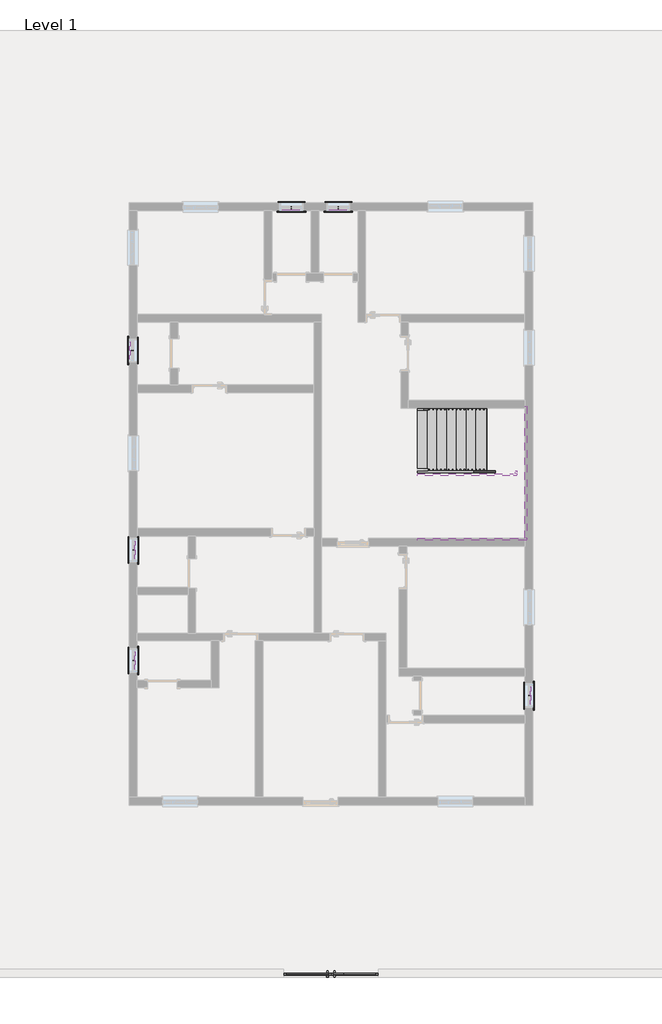
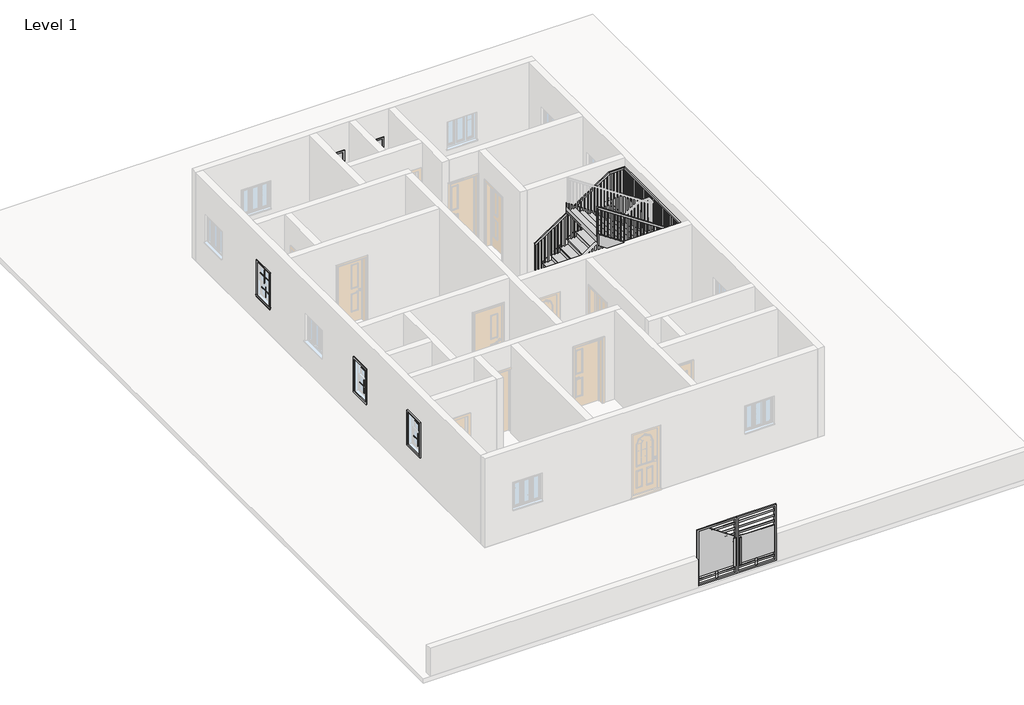
# One storey, part 3 of 3: 25 proxies, 6 members, 1 railing, 1 stair flight.
"""IFC4 building model written with IfcOpenShell, lengths in millimetres."""

from ifc_helpers import new_model, si_unit, frame, origin, place, context, project, spatial, polyline, outline, extrude, faceted_brep, transform, mapped, element, save
from components import generic_models_113f6068, muntin_pattern_2x2_muntin_pattern_2x2_eba6c5fb, trim_window_exterior_flat_with_sill_278e6a94, trim_window_interior_flat_picture_frame_e9fd5f45, stair_flight_0ebd5bc4

model = new_model("IFC4")

# Units and contexts
model_context = context("Model", 3, world=origin())
ifc_project = project(units=[si_unit("LENGTHUNIT", "METRE", prefix="MILLI")], contexts=[model_context])

# Site, building, storey
site = spatial("IfcSite", under=ifc_project)
building = spatial("IfcBuilding", under=site)
storey = spatial("IfcBuildingStorey", under=building, Name="Level 1", Elevation=0.0)

# Proxies
placement = place(None, origin())
generic_models_shape = generic_models_113f6068(model_context)
element("IfcBuildingElementProxy", 1, Name="Generic Models", at=placement, inside=storey, context=model_context, shape_type="MappedRepresentation", body=[
    mapped(generic_models_shape, transform((-8662.0711241, -2948.6655705, 0.0), x_axis=(1.0, 0.0, 0.0), y_axis=(0.0, 1.0, 0.0), z_axis=(0.0, 0.0, 1.0))),
])
muntin_pattern_2x2_muntin_pattern_2x2_shape = muntin_pattern_2x2_muntin_pattern_2x2_eba6c5fb(model_context)
element("IfcBuildingElementProxy", 2, Name="Muntin Pattern_2x2 : Muntin Pattern_2x2", ObjectType="Muntin Pattern_2x2 : Muntin Pattern_2x2", at=placement, inside=storey, context=model_context, shape_type="MappedRepresentation", body=[
    mapped(muntin_pattern_2x2_muntin_pattern_2x2_shape, transform((-13738.8961241, 8049.5344295, 1470.025), x_axis=(0.0, -1.0, 0.0), y_axis=(1.0, 0.0, 0.0), z_axis=(0.0, 0.0, 1.0))),
])
element("IfcBuildingElementProxy", 3, Name="Muntin Pattern_2x2 : Muntin Pattern_2x2", ObjectType="Muntin Pattern_2x2 : Muntin Pattern_2x2", at=placement, inside=storey, context=model_context, shape_type="MappedRepresentation", body=[
    mapped(muntin_pattern_2x2_muntin_pattern_2x2_shape, transform((-13783.3461241, 8049.5344295, 990.6), x_axis=(0.0, -1.0, 0.0), y_axis=(1.0, 0.0, 0.0), z_axis=(0.0, 0.0, 1.0))),
])
element("IfcBuildingElementProxy", 4, Name="Muntin Pattern_2x2 : Muntin Pattern_2x2", ObjectType="Muntin Pattern_2x2 : Muntin Pattern_2x2", at=placement, inside=storey, context=model_context, shape_type="MappedRepresentation", body=[
    mapped(muntin_pattern_2x2_muntin_pattern_2x2_shape, transform((-13738.8961241, 5179.3344295, 1470.025), x_axis=(0.0, -1.0, 0.0), y_axis=(1.0, 0.0, 0.0), z_axis=(0.0, 0.0, 1.0))),
])
element("IfcBuildingElementProxy", 5, Name="Muntin Pattern_2x2 : Muntin Pattern_2x2", ObjectType="Muntin Pattern_2x2 : Muntin Pattern_2x2", at=placement, inside=storey, context=model_context, shape_type="MappedRepresentation", body=[
    mapped(muntin_pattern_2x2_muntin_pattern_2x2_shape, transform((-13783.3461241, 5179.3344295, 990.6), x_axis=(0.0, -1.0, 0.0), y_axis=(1.0, 0.0, 0.0), z_axis=(0.0, 0.0, 1.0))),
])
element("IfcBuildingElementProxy", 6, Name="Muntin Pattern_2x2 : Muntin Pattern_2x2", ObjectType="Muntin Pattern_2x2 : Muntin Pattern_2x2", at=placement, inside=storey, context=model_context, shape_type="MappedRepresentation", body=[
    mapped(muntin_pattern_2x2_muntin_pattern_2x2_shape, transform((-13872.2461241, 13231.1344295, 1470.025), x_axis=(0.0, 1.0, 0.0), y_axis=(-1.0, 0.0, 0.0), z_axis=(0.0, 0.0, 1.0))),
])
element("IfcBuildingElementProxy", 7, Name="Muntin Pattern_2x2 : Muntin Pattern_2x2", ObjectType="Muntin Pattern_2x2 : Muntin Pattern_2x2", at=placement, inside=storey, context=model_context, shape_type="MappedRepresentation", body=[
    mapped(muntin_pattern_2x2_muntin_pattern_2x2_shape, transform((-13827.7961241, 13231.1344295, 990.6), x_axis=(0.0, 1.0, 0.0), y_axis=(-1.0, 0.0, 0.0), z_axis=(0.0, 0.0, 1.0))),
])
element("IfcBuildingElementProxy", 8, Name="Muntin Pattern_2x2 : Muntin Pattern_2x2", ObjectType="Muntin Pattern_2x2 : Muntin Pattern_2x2", at=placement, inside=storey, context=model_context, shape_type="MappedRepresentation", body=[
    mapped(muntin_pattern_2x2_muntin_pattern_2x2_shape, transform((-9690.7711241, 16898.2594295, 1470.025), x_axis=(-1.0, 0.0, 0.0), y_axis=(0.0, -1.0, 0.0), z_axis=(0.0, 0.0, 1.0))),
])
element("IfcBuildingElementProxy", 9, Name="Muntin Pattern_2x2 : Muntin Pattern_2x2", ObjectType="Muntin Pattern_2x2 : Muntin Pattern_2x2", at=placement, inside=storey, context=model_context, shape_type="MappedRepresentation", body=[
    mapped(muntin_pattern_2x2_muntin_pattern_2x2_shape, transform((-9690.7711241, 16942.7094295, 990.6), x_axis=(-1.0, 0.0, 0.0), y_axis=(0.0, -1.0, 0.0), z_axis=(0.0, 0.0, 1.0))),
])
element("IfcBuildingElementProxy", 10, Name="Muntin Pattern_2x2 : Muntin Pattern_2x2", ObjectType="Muntin Pattern_2x2 : Muntin Pattern_2x2", at=placement, inside=storey, context=model_context, shape_type="MappedRepresentation", body=[
    mapped(muntin_pattern_2x2_muntin_pattern_2x2_shape, transform((-8471.5711241, 16898.2594295, 1470.025), x_axis=(-1.0, 0.0, 0.0), y_axis=(0.0, -1.0, 0.0), z_axis=(0.0, 0.0, 1.0))),
])
element("IfcBuildingElementProxy", 11, Name="Muntin Pattern_2x2 : Muntin Pattern_2x2", ObjectType="Muntin Pattern_2x2 : Muntin Pattern_2x2", at=placement, inside=storey, context=model_context, shape_type="MappedRepresentation", body=[
    mapped(muntin_pattern_2x2_muntin_pattern_2x2_shape, transform((-8471.5711241, 16942.7094295, 990.6), x_axis=(-1.0, 0.0, 0.0), y_axis=(0.0, -1.0, 0.0), z_axis=(0.0, 0.0, 1.0))),
])
element("IfcBuildingElementProxy", 12, Name="Muntin Pattern_2x2 : Muntin Pattern_2x2", ObjectType="Muntin Pattern_2x2 : Muntin Pattern_2x2", at=placement, inside=storey, context=model_context, shape_type="MappedRepresentation", body=[
    mapped(muntin_pattern_2x2_muntin_pattern_2x2_shape, transform((-3451.8961241, 4264.9344295, 1470.025), x_axis=(0.0, -1.0, 0.0), y_axis=(1.0, 0.0, 0.0), z_axis=(0.0, 0.0, 1.0))),
])
element("IfcBuildingElementProxy", 13, Name="Muntin Pattern_2x2 : Muntin Pattern_2x2", ObjectType="Muntin Pattern_2x2 : Muntin Pattern_2x2", at=placement, inside=storey, context=model_context, shape_type="MappedRepresentation", body=[
    mapped(muntin_pattern_2x2_muntin_pattern_2x2_shape, transform((-3496.3461241, 4264.9344295, 990.6), x_axis=(0.0, -1.0, 0.0), y_axis=(1.0, 0.0, 0.0), z_axis=(0.0, 0.0, 1.0))),
])
trim_window_exterior_flat_with_sill_shape = trim_window_exterior_flat_with_sill_278e6a94(model_context)
element("IfcBuildingElementProxy", 14, Name="Trim-Window-Exterior-Flat : with Sill", ObjectType="Trim-Window-Exterior-Flat : with Sill", at=placement, inside=storey, context=model_context, shape_type="MappedRepresentation", body=[
    mapped(trim_window_exterior_flat_with_sill_shape, transform((-13703.9711241, 8049.5344295, 1981.2), x_axis=(0.0, 1.0, 0.0), y_axis=(0.0, 0.0, 1.0), z_axis=(1.0, 0.0, 0.0))),
])
element("IfcBuildingElementProxy", 15, Name="Trim-Window-Exterior-Flat : with Sill", ObjectType="Trim-Window-Exterior-Flat : with Sill", at=placement, inside=storey, context=model_context, shape_type="MappedRepresentation", body=[
    mapped(trim_window_exterior_flat_with_sill_shape, transform((-13703.9711241, 5179.3344295, 1981.2), x_axis=(0.0, 1.0, 0.0), y_axis=(0.0, 0.0, 1.0), z_axis=(1.0, 0.0, 0.0))),
])
element("IfcBuildingElementProxy", 16, Name="Trim-Window-Exterior-Flat : with Sill", ObjectType="Trim-Window-Exterior-Flat : with Sill", at=placement, inside=storey, context=model_context, shape_type="MappedRepresentation", body=[
    mapped(trim_window_exterior_flat_with_sill_shape, transform((-13907.1711241, 13231.1344295, 1981.2), x_axis=(0.0, -1.0, 0.0), y_axis=(0.0, 0.0, 1.0), z_axis=(-1.0, 0.0, 0.0))),
])
element("IfcBuildingElementProxy", 17, Name="Trim-Window-Exterior-Flat : with Sill", ObjectType="Trim-Window-Exterior-Flat : with Sill", at=placement, inside=storey, context=model_context, shape_type="MappedRepresentation", body=[
    mapped(trim_window_exterior_flat_with_sill_shape, transform((-9690.7711241, 16863.3344295, 1981.2), x_axis=(1.0, 0.0, 0.0), y_axis=(0.0, 0.0, 1.0), z_axis=(0.0, -1.0, 0.0))),
])
element("IfcBuildingElementProxy", 18, Name="Trim-Window-Exterior-Flat : with Sill", ObjectType="Trim-Window-Exterior-Flat : with Sill", at=placement, inside=storey, context=model_context, shape_type="MappedRepresentation", body=[
    mapped(trim_window_exterior_flat_with_sill_shape, transform((-8471.5711241, 16863.3344295, 1981.2), x_axis=(1.0, 0.0, 0.0), y_axis=(0.0, 0.0, 1.0), z_axis=(0.0, -1.0, 0.0))),
])
element("IfcBuildingElementProxy", 19, Name="Trim-Window-Exterior-Flat : with Sill", ObjectType="Trim-Window-Exterior-Flat : with Sill", at=placement, inside=storey, context=model_context, shape_type="MappedRepresentation", body=[
    mapped(trim_window_exterior_flat_with_sill_shape, transform((-3416.9711241, 4264.9344295, 1981.2), x_axis=(0.0, 1.0, 0.0), y_axis=(0.0, 0.0, 1.0), z_axis=(1.0, 0.0, 0.0))),
])
trim_window_interior_flat_picture_frame_shape = trim_window_interior_flat_picture_frame_e9fd5f45(model_context)
element("IfcBuildingElementProxy", 20, Name="Trim-Window-Interior-Flat : Picture Frame", ObjectType="Trim-Window-Interior-Flat : Picture Frame", at=placement, inside=storey, context=model_context, shape_type="MappedRepresentation", body=[
    mapped(trim_window_interior_flat_picture_frame_shape, transform((-13907.1711241, 8049.5344295, 1981.2), x_axis=(0.0, -1.0, 0.0), y_axis=(0.0, 0.0, 1.0), z_axis=(-1.0, 0.0, 0.0))),
])
element("IfcBuildingElementProxy", 21, Name="Trim-Window-Interior-Flat : Picture Frame", ObjectType="Trim-Window-Interior-Flat : Picture Frame", at=placement, inside=storey, context=model_context, shape_type="MappedRepresentation", body=[
    mapped(trim_window_interior_flat_picture_frame_shape, transform((-13907.1711241, 5179.3344295, 1981.2), x_axis=(0.0, -1.0, 0.0), y_axis=(0.0, 0.0, 1.0), z_axis=(-1.0, 0.0, 0.0))),
])
element("IfcBuildingElementProxy", 22, Name="Trim-Window-Interior-Flat : Picture Frame", ObjectType="Trim-Window-Interior-Flat : Picture Frame", at=placement, inside=storey, context=model_context, shape_type="MappedRepresentation", body=[
    mapped(trim_window_interior_flat_picture_frame_shape, transform((-13703.9711241, 13231.1344295, 1981.2), x_axis=(0.0, 1.0, 0.0), y_axis=(0.0, 0.0, 1.0), z_axis=(1.0, 0.0, 0.0))),
])
element("IfcBuildingElementProxy", 23, Name="Trim-Window-Interior-Flat : Picture Frame", ObjectType="Trim-Window-Interior-Flat : Picture Frame", at=placement, inside=storey, context=model_context, shape_type="MappedRepresentation", body=[
    mapped(trim_window_interior_flat_picture_frame_shape, transform((-9690.7711241, 17066.5344295, 1981.2), x_axis=(-1.0, 0.0, 0.0), y_axis=(0.0, 0.0, 1.0), z_axis=(0.0, 1.0, 0.0))),
])
element("IfcBuildingElementProxy", 24, Name="Trim-Window-Interior-Flat : Picture Frame", ObjectType="Trim-Window-Interior-Flat : Picture Frame", at=placement, inside=storey, context=model_context, shape_type="MappedRepresentation", body=[
    mapped(trim_window_interior_flat_picture_frame_shape, transform((-8471.5711241, 17066.5344295, 1981.2), x_axis=(-1.0, 0.0, 0.0), y_axis=(0.0, 0.0, 1.0), z_axis=(0.0, 1.0, 0.0))),
])
element("IfcBuildingElementProxy", 25, Name="Trim-Window-Interior-Flat : Picture Frame", ObjectType="Trim-Window-Interior-Flat : Picture Frame", at=placement, inside=storey, context=model_context, shape_type="MappedRepresentation", body=[
    mapped(trim_window_interior_flat_picture_frame_shape, transform((-3620.1711241, 4264.9344295, 1981.2), x_axis=(0.0, -1.0, 0.0), y_axis=(0.0, 0.0, 1.0), z_axis=(-1.0, 0.0, 0.0))),
])

# Members
element("IfcMember", 26, ObjectType="Stringer - 2\" Width", at=placement, inside=storey, context=model_context, shape_type="SweptSolid", body=[
    extrude(outline(polyline([(218.0398409, -6414.1711241), (0.0, -6414.1711241), (0.0, -6191.7448711), (1714.382498, -3620.1711241), (1769.5333333, -3620.1711241), (1769.5333333, -4086.9308855), (218.0398409, -6414.1711241)])), frame((0.0, 11732.5344295, 0.0), z_axis=(0.0, 1.0, 0.0), x_axis=(0.0, 0.0, 1.0)), (0.0, 0.0, 1.0), 50.8),
])
element("IfcMember", 27, ObjectType="Stringer - 2\" Width", at=placement, inside=storey, context=model_context, shape_type="SweptSolid", body=[
    extrude(outline(polyline([(-3620.1711241, 11783.3344295), (-3569.3711241, 11783.3344295), (-3569.3711241, 8354.3344295), (-3620.1711241, 8354.3344295), (-3620.1711241, 11783.3344295)])), frame((0.0, 0.0, 1464.7333333), z_axis=(0.0, 0.0, 1.0), x_axis=(1.0, 0.0, 0.0)), (0.0, 0.0, 1.0), 304.8),
])
element("IfcMember", 28, ObjectType="Stringer - 2\" Width", at=placement, inside=storey, context=model_context, shape_type="SweptSolid", body=[
    extrude(outline(polyline([(1464.7333333, -3569.3711241), (1538.8398409, -3569.3711241), (3435.3731743, -6414.1711241), (3069.0491647, -6414.1711241), (1464.7333333, -4007.6973771), (1464.7333333, -3569.3711241)])), frame((0.0, 8303.5344295, 0.0), z_axis=(0.0, 1.0, 0.0), x_axis=(0.0, 0.0, 1.0)), (0.0, 0.0, 1.0), 50.8),
])
element("IfcMember", 29, ObjectType="Stringer - 2\" Width", at=placement, inside=storey, context=model_context, shape_type="SweptSolid", body=[
    extrude(outline(polyline([(218.0398409, -6414.1711241), (0.0, -6414.1711241), (0.0, -6191.7448711), (1545.0491647, -3874.1711241), (1769.5333333, -3874.1711241), (1769.5333333, -4086.9308855), (218.0398409, -6414.1711241)])), frame((0.0, 10056.1344295, 0.0), z_axis=(0.0, 1.0, 0.0), x_axis=(0.0, 0.0, 1.0)), (0.0, 0.0, 1.0), 50.8),
])
element("IfcMember", 30, ObjectType="Stringer - 2\" Width", at=placement, inside=storey, context=model_context, shape_type="SweptSolid", body=[
    extrude(outline(polyline([(-3874.1711241, 10106.9344295), (-3823.3711241, 10106.9344295), (-3823.3711241, 10030.7344295), (-3874.1711241, 10030.7344295), (-3874.1711241, 10106.9344295)])), frame((0.0, 0.0, 1464.7333333), z_axis=(0.0, 0.0, 1.0), x_axis=(1.0, 0.0, 0.0)), (0.0, 0.0, 1.0), 304.8),
])
element("IfcMember", 31, ObjectType="Stringer - 2\" Width", at=placement, inside=storey, context=model_context, shape_type="SweptSolid", body=[
    extrude(outline(polyline([(1464.7333333, -3823.3711241), (1708.1731743, -3823.3711241), (3435.3731743, -6414.1711241), (3069.0491647, -6414.1711241), (1464.7333333, -4007.6973771), (1464.7333333, -3823.3711241)])), frame((0.0, 9979.9344295, 0.0), z_axis=(0.0, 1.0, 0.0), x_axis=(0.0, 0.0, 1.0)), (0.0, 0.0, 1.0), 50.8),
])

# Railing
element("IfcRailing", 32, ObjectType="Handrail - Rectangular", at=placement, inside=storey, context=model_context, shape_type="SolidModel", body=[
    faceted_brep([(-6414.1711241, 11732.5344295, 1083.7333333), (-6414.1711241, 11732.5344295, 1022.6793317), (-6414.1711241, 11681.7344295, 1022.6793317), (-6414.1711241, 11681.7344295, 1083.7333333), (-4128.1711241, 11732.5344295, 2607.7333333), (-4112.7901217, 11732.5344295, 2556.9333333), (-4112.7901217, 11681.7344295, 2556.9333333), (-4128.1711241, 11681.7344295, 2607.7333333), (-3620.1711241, 11732.5344295, 2607.7333333), (-3620.1711241, 11732.5344295, 2556.9333333), (-3670.9711241, 11681.7344295, 2556.9333333), (-3670.9711241, 11681.7344295, 2607.7333333), (-3620.1711241, 8354.3344295, 2607.7333333), (-3620.1711241, 8354.3344295, 2556.9333333), (-3670.9711241, 8405.1344295, 2556.9333333), (-3670.9711241, 8405.1344295, 2607.7333333), (-3874.1711241, 8354.3344295, 2607.7333333), (-3889.5521265, 8354.3344295, 2556.9333333), (-3889.5521265, 8405.1344295, 2556.9333333), (-3874.1711241, 8405.1344295, 2607.7333333), (-6414.1711241, 8354.3344295, 4301.0666667), (-6414.1711241, 8405.1344295, 4301.0666667), (-6414.1711241, 8405.1344295, 4240.0126651), (-6414.1711241, 8354.3344295, 4240.0126651)], [[[0, 1, 2, 3]], [[1, 0, 4, 5]], [[2, 1, 5, 6]], [[3, 2, 6, 7]], [[0, 3, 7, 4]], [[5, 4, 8, 9]], [[6, 5, 9, 10]], [[7, 6, 10, 11]], [[4, 7, 11, 8]], [[9, 8, 12, 13]], [[10, 9, 13, 14]], [[11, 10, 14, 15]], [[8, 11, 15, 12]], [[13, 12, 16, 17]], [[14, 13, 17, 18]], [[15, 14, 18, 19]], [[12, 15, 19, 16]], [[20, 21, 22, 23]], [[17, 16, 20, 23]], [[18, 17, 23, 22]], [[19, 18, 22, 21]], [[16, 19, 21, 20]]]),
    extrude(outline(polyline([(4229.4293317, -6398.2961241), (3217.3333333, -6398.2961241), (3217.3333333, -6379.2461241), (4216.7293317, -6379.2461241), (4229.4293317, -6398.2961241)])), frame((0.0, 8370.2094295, 0.0), z_axis=(0.0, 1.0, 0.0), x_axis=(0.0, 0.0, 1.0)), (0.0, 0.0, 1.0), 19.05),
    extrude(outline(polyline([(4161.6959984, -6296.6961241), (3217.3333333, -6296.6961241), (3217.3333333, -6277.6461241), (4148.9959984, -6277.6461241), (4161.6959984, -6296.6961241)])), frame((0.0, 8370.2094295, 0.0), z_axis=(0.0, 1.0, 0.0), x_axis=(0.0, 0.0, 1.0)), (0.0, 0.0, 1.0), 19.05),
    extrude(outline(polyline([(4093.9626651, -6195.0961241), (3217.3333333, -6195.0961241), (3217.3333333, -6176.0461241), (4081.2626651, -6176.0461241), (4093.9626651, -6195.0961241)])), frame((0.0, 8370.2094295, 0.0), z_axis=(0.0, 1.0, 0.0), x_axis=(0.0, 0.0, 1.0)), (0.0, 0.0, 1.0), 19.05),
    extrude(outline(polyline([(4026.2293317, -6093.4961241), (3048.0, -6093.4961241), (3048.0, -6074.4461241), (4013.5293317, -6074.4461241), (4026.2293317, -6093.4961241)])), frame((0.0, 8370.2094295, 0.0), z_axis=(0.0, 1.0, 0.0), x_axis=(0.0, 0.0, 1.0)), (0.0, 0.0, 1.0), 19.05),
    extrude(outline(polyline([(3958.4959984, -5991.8961241), (3048.0, -5991.8961241), (3048.0, -5972.8461241), (3945.7959984, -5972.8461241), (3958.4959984, -5991.8961241)])), frame((0.0, 8370.2094295, 0.0), z_axis=(0.0, 1.0, 0.0), x_axis=(0.0, 0.0, 1.0)), (0.0, 0.0, 1.0), 19.05),
    extrude(outline(polyline([(3890.7626651, -5890.2961241), (2878.6666667, -5890.2961241), (2878.6666667, -5871.2461241), (3878.0626651, -5871.2461241), (3890.7626651, -5890.2961241)])), frame((0.0, 8370.2094295, 0.0), z_axis=(0.0, 1.0, 0.0), x_axis=(0.0, 0.0, 1.0)), (0.0, 0.0, 1.0), 19.05),
    extrude(outline(polyline([(3823.0293317, -5788.6961241), (2878.6666667, -5788.6961241), (2878.6666667, -5769.6461241), (3810.3293317, -5769.6461241), (3823.0293317, -5788.6961241)])), frame((0.0, 8370.2094295, 0.0), z_axis=(0.0, 1.0, 0.0), x_axis=(0.0, 0.0, 1.0)), (0.0, 0.0, 1.0), 19.05),
    extrude(outline(polyline([(3755.2959984, -5687.0961241), (2878.6666667, -5687.0961241), (2878.6666667, -5668.0461241), (3742.5959984, -5668.0461241), (3755.2959984, -5687.0961241)])), frame((0.0, 8370.2094295, 0.0), z_axis=(0.0, 1.0, 0.0), x_axis=(0.0, 0.0, 1.0)), (0.0, 0.0, 1.0), 19.05),
    extrude(outline(polyline([(3687.5626651, -5585.4961241), (2709.3333333, -5585.4961241), (2709.3333333, -5566.4461241), (3674.8626651, -5566.4461241), (3687.5626651, -5585.4961241)])), frame((0.0, 8370.2094295, 0.0), z_axis=(0.0, 1.0, 0.0), x_axis=(0.0, 0.0, 1.0)), (0.0, 0.0, 1.0), 19.05),
    extrude(outline(polyline([(3619.8293317, -5483.8961241), (2709.3333333, -5483.8961241), (2709.3333333, -5464.8461241), (3607.1293317, -5464.8461241), (3619.8293317, -5483.8961241)])), frame((0.0, 8370.2094295, 0.0), z_axis=(0.0, 1.0, 0.0), x_axis=(0.0, 0.0, 1.0)), (0.0, 0.0, 1.0), 19.05),
    extrude(outline(polyline([(3552.0959984, -5382.2961241), (2540.0, -5382.2961241), (2540.0, -5363.2461241), (3539.3959984, -5363.2461241), (3552.0959984, -5382.2961241)])), frame((0.0, 8370.2094295, 0.0), z_axis=(0.0, 1.0, 0.0), x_axis=(0.0, 0.0, 1.0)), (0.0, 0.0, 1.0), 19.05),
    extrude(outline(polyline([(3484.3626651, -5280.6961241), (2540.0, -5280.6961241), (2540.0, -5261.6461241), (3471.6626651, -5261.6461241), (3484.3626651, -5280.6961241)])), frame((0.0, 8370.2094295, 0.0), z_axis=(0.0, 1.0, 0.0), x_axis=(0.0, 0.0, 1.0)), (0.0, 0.0, 1.0), 19.05),
    extrude(outline(polyline([(3416.6293317, -5179.0961241), (2540.0, -5179.0961241), (2540.0, -5160.0461241), (3403.9293317, -5160.0461241), (3416.6293317, -5179.0961241)])), frame((0.0, 8370.2094295, 0.0), z_axis=(0.0, 1.0, 0.0), x_axis=(0.0, 0.0, 1.0)), (0.0, 0.0, 1.0), 19.05),
    extrude(outline(polyline([(3348.8959984, -5077.4961241), (2370.6666667, -5077.4961241), (2370.6666667, -5058.4461241), (3336.1959984, -5058.4461241), (3348.8959984, -5077.4961241)])), frame((0.0, 8370.2094295, 0.0), z_axis=(0.0, 1.0, 0.0), x_axis=(0.0, 0.0, 1.0)), (0.0, 0.0, 1.0), 19.05),
    extrude(outline(polyline([(3281.1626651, -4975.8961241), (2370.6666667, -4975.8961241), (2370.6666667, -4956.8461241), (3268.4626651, -4956.8461241), (3281.1626651, -4975.8961241)])), frame((0.0, 8370.2094295, 0.0), z_axis=(0.0, 1.0, 0.0), x_axis=(0.0, 0.0, 1.0)), (0.0, 0.0, 1.0), 19.05),
    extrude(outline(polyline([(3213.4293317, -4874.2961241), (2201.3333333, -4874.2961241), (2201.3333333, -4855.2461241), (3200.7293317, -4855.2461241), (3213.4293317, -4874.2961241)])), frame((0.0, 8370.2094295, 0.0), z_axis=(0.0, 1.0, 0.0), x_axis=(0.0, 0.0, 1.0)), (0.0, 0.0, 1.0), 19.05),
    extrude(outline(polyline([(3145.6959984, -4772.6961241), (2201.3333333, -4772.6961241), (2201.3333333, -4753.6461241), (3132.9959984, -4753.6461241), (3145.6959984, -4772.6961241)])), frame((0.0, 8370.2094295, 0.0), z_axis=(0.0, 1.0, 0.0), x_axis=(0.0, 0.0, 1.0)), (0.0, 0.0, 1.0), 19.05),
    extrude(outline(polyline([(3077.9626651, -4671.0961241), (2201.3333333, -4671.0961241), (2201.3333333, -4652.0461241), (3065.2626651, -4652.0461241), (3077.9626651, -4671.0961241)])), frame((0.0, 8370.2094295, 0.0), z_axis=(0.0, 1.0, 0.0), x_axis=(0.0, 0.0, 1.0)), (0.0, 0.0, 1.0), 19.05),
    extrude(outline(polyline([(3010.2293317, -4569.4961241), (2032.0, -4569.4961241), (2032.0, -4550.4461241), (2997.5293317, -4550.4461241), (3010.2293317, -4569.4961241)])), frame((0.0, 8370.2094295, 0.0), z_axis=(0.0, 1.0, 0.0), x_axis=(0.0, 0.0, 1.0)), (0.0, 0.0, 1.0), 19.05),
    extrude(outline(polyline([(2942.4959984, -4467.8961241), (2032.0, -4467.8961241), (2032.0, -4448.8461241), (2929.7959984, -4448.8461241), (2942.4959984, -4467.8961241)])), frame((0.0, 8370.2094295, 0.0), z_axis=(0.0, 1.0, 0.0), x_axis=(0.0, 0.0, 1.0)), (0.0, 0.0, 1.0), 19.05),
    extrude(outline(polyline([(2874.7626651, -4366.2961241), (1862.6666667, -4366.2961241), (1862.6666667, -4347.2461241), (2862.0626651, -4347.2461241), (2874.7626651, -4366.2961241)])), frame((0.0, 8370.2094295, 0.0), z_axis=(0.0, 1.0, 0.0), x_axis=(0.0, 0.0, 1.0)), (0.0, 0.0, 1.0), 19.05),
    extrude(outline(polyline([(2807.0293317, -4264.6961241), (1862.6666667, -4264.6961241), (1862.6666667, -4245.6461241), (2794.3293317, -4245.6461241), (2807.0293317, -4264.6961241)])), frame((0.0, 8370.2094295, 0.0), z_axis=(0.0, 1.0, 0.0), x_axis=(0.0, 0.0, 1.0)), (0.0, 0.0, 1.0), 19.05),
    extrude(outline(polyline([(2739.2959984, -4163.0961241), (1862.6666667, -4163.0961241), (1862.6666667, -4144.0461241), (2726.5959984, -4144.0461241), (2739.2959984, -4163.0961241)])), frame((0.0, 8370.2094295, 0.0), z_axis=(0.0, 1.0, 0.0), x_axis=(0.0, 0.0, 1.0)), (0.0, 0.0, 1.0), 19.05),
    extrude(outline(polyline([(2671.5626651, -4061.4961241), (1693.3333333, -4061.4961241), (1693.3333333, -4042.4461241), (2658.8626651, -4042.4461241), (2671.5626651, -4061.4961241)])), frame((0.0, 8370.2094295, 0.0), z_axis=(0.0, 1.0, 0.0), x_axis=(0.0, 0.0, 1.0)), (0.0, 0.0, 1.0), 19.05),
    extrude(outline(polyline([(2603.8293317, -3959.8961241), (1693.3333333, -3959.8961241), (1693.3333333, -3940.8461241), (2591.1293317, -3940.8461241), (2603.8293317, -3959.8961241)])), frame((0.0, 8370.2094295, 0.0), z_axis=(0.0, 1.0, 0.0), x_axis=(0.0, 0.0, 1.0)), (0.0, 0.0, 1.0), 19.05),
    extrude(outline(polyline([(-3839.2461241, 8370.2094295), (-3858.2961241, 8370.2094295), (-3858.2961241, 8389.2594295), (-3839.2461241, 8389.2594295), (-3839.2461241, 8370.2094295)])), frame((0.0, 0.0, 1693.3333333), z_axis=(0.0, 0.0, 1.0), x_axis=(1.0, 0.0, 0.0)), (0.0, 0.0, 1.0), 863.6),
    extrude(outline(polyline([(-3737.6461241, 8370.2094295), (-3756.6961241, 8370.2094295), (-3756.6961241, 8389.2594295), (-3737.6461241, 8389.2594295), (-3737.6461241, 8370.2094295)])), frame((0.0, 0.0, 1693.3333333), z_axis=(0.0, 0.0, 1.0), x_axis=(1.0, 0.0, 0.0)), (0.0, 0.0, 1.0), 863.6),
    extrude(outline(polyline([(-3636.0461241, 8465.4594295), (-3636.0461241, 8446.4094295), (-3655.0961241, 8446.4094295), (-3655.0961241, 8465.4594295), (-3636.0461241, 8465.4594295)])), frame((0.0, 0.0, 1693.3333333), z_axis=(0.0, 0.0, 1.0), x_axis=(1.0, 0.0, 0.0)), (0.0, 0.0, 1.0), 863.6),
    extrude(outline(polyline([(-3636.0461241, 8567.0594295), (-3636.0461241, 8548.0094295), (-3655.0961241, 8548.0094295), (-3655.0961241, 8567.0594295), (-3636.0461241, 8567.0594295)])), frame((0.0, 0.0, 1693.3333333), z_axis=(0.0, 0.0, 1.0), x_axis=(1.0, 0.0, 0.0)), (0.0, 0.0, 1.0), 863.6),
    extrude(outline(polyline([(-3636.0461241, 8668.6594295), (-3636.0461241, 8649.6094295), (-3655.0961241, 8649.6094295), (-3655.0961241, 8668.6594295), (-3636.0461241, 8668.6594295)])), frame((0.0, 0.0, 1693.3333333), z_axis=(0.0, 0.0, 1.0), x_axis=(1.0, 0.0, 0.0)), (0.0, 0.0, 1.0), 863.6),
    extrude(outline(polyline([(-3636.0461241, 8770.2594295), (-3636.0461241, 8751.2094295), (-3655.0961241, 8751.2094295), (-3655.0961241, 8770.2594295), (-3636.0461241, 8770.2594295)])), frame((0.0, 0.0, 1693.3333333), z_axis=(0.0, 0.0, 1.0), x_axis=(1.0, 0.0, 0.0)), (0.0, 0.0, 1.0), 863.6),
    extrude(outline(polyline([(-3636.0461241, 8871.8594295), (-3636.0461241, 8852.8094295), (-3655.0961241, 8852.8094295), (-3655.0961241, 8871.8594295), (-3636.0461241, 8871.8594295)])), frame((0.0, 0.0, 1693.3333333), z_axis=(0.0, 0.0, 1.0), x_axis=(1.0, 0.0, 0.0)), (0.0, 0.0, 1.0), 863.6),
    extrude(outline(polyline([(-3636.0461241, 8973.4594295), (-3636.0461241, 8954.4094295), (-3655.0961241, 8954.4094295), (-3655.0961241, 8973.4594295), (-3636.0461241, 8973.4594295)])), frame((0.0, 0.0, 1693.3333333), z_axis=(0.0, 0.0, 1.0), x_axis=(1.0, 0.0, 0.0)), (0.0, 0.0, 1.0), 863.6),
    extrude(outline(polyline([(-3636.0461241, 9075.0594295), (-3636.0461241, 9056.0094295), (-3655.0961241, 9056.0094295), (-3655.0961241, 9075.0594295), (-3636.0461241, 9075.0594295)])), frame((0.0, 0.0, 1693.3333333), z_axis=(0.0, 0.0, 1.0), x_axis=(1.0, 0.0, 0.0)), (0.0, 0.0, 1.0), 863.6),
    extrude(outline(polyline([(-3636.0461241, 9176.6594295), (-3636.0461241, 9157.6094295), (-3655.0961241, 9157.6094295), (-3655.0961241, 9176.6594295), (-3636.0461241, 9176.6594295)])), frame((0.0, 0.0, 1693.3333333), z_axis=(0.0, 0.0, 1.0), x_axis=(1.0, 0.0, 0.0)), (0.0, 0.0, 1.0), 863.6),
    extrude(outline(polyline([(-3636.0461241, 9278.2594295), (-3636.0461241, 9259.2094295), (-3655.0961241, 9259.2094295), (-3655.0961241, 9278.2594295), (-3636.0461241, 9278.2594295)])), frame((0.0, 0.0, 1693.3333333), z_axis=(0.0, 0.0, 1.0), x_axis=(1.0, 0.0, 0.0)), (0.0, 0.0, 1.0), 863.6),
    extrude(outline(polyline([(-3636.0461241, 9379.8594295), (-3636.0461241, 9360.8094295), (-3655.0961241, 9360.8094295), (-3655.0961241, 9379.8594295), (-3636.0461241, 9379.8594295)])), frame((0.0, 0.0, 1693.3333333), z_axis=(0.0, 0.0, 1.0), x_axis=(1.0, 0.0, 0.0)), (0.0, 0.0, 1.0), 863.6),
    extrude(outline(polyline([(-3636.0461241, 9481.4594295), (-3636.0461241, 9462.4094295), (-3655.0961241, 9462.4094295), (-3655.0961241, 9481.4594295), (-3636.0461241, 9481.4594295)])), frame((0.0, 0.0, 1693.3333333), z_axis=(0.0, 0.0, 1.0), x_axis=(1.0, 0.0, 0.0)), (0.0, 0.0, 1.0), 863.6),
    extrude(outline(polyline([(-3636.0461241, 9583.0594295), (-3636.0461241, 9564.0094295), (-3655.0961241, 9564.0094295), (-3655.0961241, 9583.0594295), (-3636.0461241, 9583.0594295)])), frame((0.0, 0.0, 1693.3333333), z_axis=(0.0, 0.0, 1.0), x_axis=(1.0, 0.0, 0.0)), (0.0, 0.0, 1.0), 863.6),
    extrude(outline(polyline([(-3636.0461241, 9684.6594295), (-3636.0461241, 9665.6094295), (-3655.0961241, 9665.6094295), (-3655.0961241, 9684.6594295), (-3636.0461241, 9684.6594295)])), frame((0.0, 0.0, 1693.3333333), z_axis=(0.0, 0.0, 1.0), x_axis=(1.0, 0.0, 0.0)), (0.0, 0.0, 1.0), 863.6),
    extrude(outline(polyline([(-3636.0461241, 9786.2594295), (-3636.0461241, 9767.2094295), (-3655.0961241, 9767.2094295), (-3655.0961241, 9786.2594295), (-3636.0461241, 9786.2594295)])), frame((0.0, 0.0, 1693.3333333), z_axis=(0.0, 0.0, 1.0), x_axis=(1.0, 0.0, 0.0)), (0.0, 0.0, 1.0), 863.6),
    extrude(outline(polyline([(-3636.0461241, 9887.8594295), (-3636.0461241, 9868.8094295), (-3655.0961241, 9868.8094295), (-3655.0961241, 9887.8594295), (-3636.0461241, 9887.8594295)])), frame((0.0, 0.0, 1693.3333333), z_axis=(0.0, 0.0, 1.0), x_axis=(1.0, 0.0, 0.0)), (0.0, 0.0, 1.0), 863.6),
    extrude(outline(polyline([(-3636.0461241, 9989.4594295), (-3636.0461241, 9970.4094295), (-3655.0961241, 9970.4094295), (-3655.0961241, 9989.4594295), (-3636.0461241, 9989.4594295)])), frame((0.0, 0.0, 1693.3333333), z_axis=(0.0, 0.0, 1.0), x_axis=(1.0, 0.0, 0.0)), (0.0, 0.0, 1.0), 863.6),
    extrude(outline(polyline([(-3636.0461241, 10091.0594295), (-3636.0461241, 10072.0094295), (-3655.0961241, 10072.0094295), (-3655.0961241, 10091.0594295), (-3636.0461241, 10091.0594295)])), frame((0.0, 0.0, 1693.3333333), z_axis=(0.0, 0.0, 1.0), x_axis=(1.0, 0.0, 0.0)), (0.0, 0.0, 1.0), 863.6),
    extrude(outline(polyline([(-3636.0461241, 10192.6594295), (-3636.0461241, 10173.6094295), (-3655.0961241, 10173.6094295), (-3655.0961241, 10192.6594295), (-3636.0461241, 10192.6594295)])), frame((0.0, 0.0, 1693.3333333), z_axis=(0.0, 0.0, 1.0), x_axis=(1.0, 0.0, 0.0)), (0.0, 0.0, 1.0), 863.6),
    extrude(outline(polyline([(-3636.0461241, 10294.2594295), (-3636.0461241, 10275.2094295), (-3655.0961241, 10275.2094295), (-3655.0961241, 10294.2594295), (-3636.0461241, 10294.2594295)])), frame((0.0, 0.0, 1693.3333333), z_axis=(0.0, 0.0, 1.0), x_axis=(1.0, 0.0, 0.0)), (0.0, 0.0, 1.0), 863.6),
    extrude(outline(polyline([(-3636.0461241, 10395.8594295), (-3636.0461241, 10376.8094295), (-3655.0961241, 10376.8094295), (-3655.0961241, 10395.8594295), (-3636.0461241, 10395.8594295)])), frame((0.0, 0.0, 1693.3333333), z_axis=(0.0, 0.0, 1.0), x_axis=(1.0, 0.0, 0.0)), (0.0, 0.0, 1.0), 863.6),
    extrude(outline(polyline([(-3636.0461241, 10497.4594295), (-3636.0461241, 10478.4094295), (-3655.0961241, 10478.4094295), (-3655.0961241, 10497.4594295), (-3636.0461241, 10497.4594295)])), frame((0.0, 0.0, 1693.3333333), z_axis=(0.0, 0.0, 1.0), x_axis=(1.0, 0.0, 0.0)), (0.0, 0.0, 1.0), 863.6),
    extrude(outline(polyline([(-3636.0461241, 10599.0594295), (-3636.0461241, 10580.0094295), (-3655.0961241, 10580.0094295), (-3655.0961241, 10599.0594295), (-3636.0461241, 10599.0594295)])), frame((0.0, 0.0, 1693.3333333), z_axis=(0.0, 0.0, 1.0), x_axis=(1.0, 0.0, 0.0)), (0.0, 0.0, 1.0), 863.6),
    extrude(outline(polyline([(-3636.0461241, 10700.6594295), (-3636.0461241, 10681.6094295), (-3655.0961241, 10681.6094295), (-3655.0961241, 10700.6594295), (-3636.0461241, 10700.6594295)])), frame((0.0, 0.0, 1693.3333333), z_axis=(0.0, 0.0, 1.0), x_axis=(1.0, 0.0, 0.0)), (0.0, 0.0, 1.0), 863.6),
    extrude(outline(polyline([(-3636.0461241, 10802.2594295), (-3636.0461241, 10783.2094295), (-3655.0961241, 10783.2094295), (-3655.0961241, 10802.2594295), (-3636.0461241, 10802.2594295)])), frame((0.0, 0.0, 1693.3333333), z_axis=(0.0, 0.0, 1.0), x_axis=(1.0, 0.0, 0.0)), (0.0, 0.0, 1.0), 863.6),
    extrude(outline(polyline([(-3636.0461241, 10903.8594295), (-3636.0461241, 10884.8094295), (-3655.0961241, 10884.8094295), (-3655.0961241, 10903.8594295), (-3636.0461241, 10903.8594295)])), frame((0.0, 0.0, 1693.3333333), z_axis=(0.0, 0.0, 1.0), x_axis=(1.0, 0.0, 0.0)), (0.0, 0.0, 1.0), 863.6),
    extrude(outline(polyline([(-3636.0461241, 11005.4594295), (-3636.0461241, 10986.4094295), (-3655.0961241, 10986.4094295), (-3655.0961241, 11005.4594295), (-3636.0461241, 11005.4594295)])), frame((0.0, 0.0, 1693.3333333), z_axis=(0.0, 0.0, 1.0), x_axis=(1.0, 0.0, 0.0)), (0.0, 0.0, 1.0), 863.6),
    extrude(outline(polyline([(-3636.0461241, 11107.0594295), (-3636.0461241, 11088.0094295), (-3655.0961241, 11088.0094295), (-3655.0961241, 11107.0594295), (-3636.0461241, 11107.0594295)])), frame((0.0, 0.0, 1693.3333333), z_axis=(0.0, 0.0, 1.0), x_axis=(1.0, 0.0, 0.0)), (0.0, 0.0, 1.0), 863.6),
    extrude(outline(polyline([(-3636.0461241, 11208.6594295), (-3636.0461241, 11189.6094295), (-3655.0961241, 11189.6094295), (-3655.0961241, 11208.6594295), (-3636.0461241, 11208.6594295)])), frame((0.0, 0.0, 1693.3333333), z_axis=(0.0, 0.0, 1.0), x_axis=(1.0, 0.0, 0.0)), (0.0, 0.0, 1.0), 863.6),
    extrude(outline(polyline([(-3636.0461241, 11310.2594295), (-3636.0461241, 11291.2094295), (-3655.0961241, 11291.2094295), (-3655.0961241, 11310.2594295), (-3636.0461241, 11310.2594295)])), frame((0.0, 0.0, 1693.3333333), z_axis=(0.0, 0.0, 1.0), x_axis=(1.0, 0.0, 0.0)), (0.0, 0.0, 1.0), 863.6),
    extrude(outline(polyline([(-3636.0461241, 11411.8594295), (-3636.0461241, 11392.8094295), (-3655.0961241, 11392.8094295), (-3655.0961241, 11411.8594295), (-3636.0461241, 11411.8594295)])), frame((0.0, 0.0, 1693.3333333), z_axis=(0.0, 0.0, 1.0), x_axis=(1.0, 0.0, 0.0)), (0.0, 0.0, 1.0), 863.6),
    extrude(outline(polyline([(-3636.0461241, 11513.4594295), (-3636.0461241, 11494.4094295), (-3655.0961241, 11494.4094295), (-3655.0961241, 11513.4594295), (-3636.0461241, 11513.4594295)])), frame((0.0, 0.0, 1693.3333333), z_axis=(0.0, 0.0, 1.0), x_axis=(1.0, 0.0, 0.0)), (0.0, 0.0, 1.0), 863.6),
    extrude(outline(polyline([(-3636.0461241, 11615.0594295), (-3636.0461241, 11596.0094295), (-3655.0961241, 11596.0094295), (-3655.0961241, 11615.0594295), (-3636.0461241, 11615.0594295)])), frame((0.0, 0.0, 1693.3333333), z_axis=(0.0, 0.0, 1.0), x_axis=(1.0, 0.0, 0.0)), (0.0, 0.0, 1.0), 863.6),
    extrude(outline(polyline([(-3680.4961241, 11716.6594295), (-3661.4461241, 11716.6594295), (-3661.4461241, 11697.6094295), (-3680.4961241, 11697.6094295), (-3680.4961241, 11716.6594295)])), frame((0.0, 0.0, 1693.3333333), z_axis=(0.0, 0.0, 1.0), x_axis=(1.0, 0.0, 0.0)), (0.0, 0.0, 1.0), 863.6),
    extrude(outline(polyline([(-3782.0961241, 11716.6594295), (-3763.0461241, 11716.6594295), (-3763.0461241, 11697.6094295), (-3782.0961241, 11697.6094295), (-3782.0961241, 11716.6594295)])), frame((0.0, 0.0, 1693.3333333), z_axis=(0.0, 0.0, 1.0), x_axis=(1.0, 0.0, 0.0)), (0.0, 0.0, 1.0), 863.6),
    extrude(outline(polyline([(-3883.6961241, 11716.6594295), (-3864.6461241, 11716.6594295), (-3864.6461241, 11697.6094295), (-3883.6961241, 11697.6094295), (-3883.6961241, 11716.6594295)])), frame((0.0, 0.0, 1693.3333333), z_axis=(0.0, 0.0, 1.0), x_axis=(1.0, 0.0, 0.0)), (0.0, 0.0, 1.0), 863.6),
    extrude(outline(polyline([(-3985.2961241, 11716.6594295), (-3966.2461241, 11716.6594295), (-3966.2461241, 11697.6094295), (-3985.2961241, 11697.6094295), (-3985.2961241, 11716.6594295)])), frame((0.0, 0.0, 1693.3333333), z_axis=(0.0, 0.0, 1.0), x_axis=(1.0, 0.0, 0.0)), (0.0, 0.0, 1.0), 863.6),
    extrude(outline(polyline([(-4086.8961241, 11716.6594295), (-4067.8461241, 11716.6594295), (-4067.8461241, 11697.6094295), (-4086.8961241, 11697.6094295), (-4086.8961241, 11716.6594295)])), frame((0.0, 0.0, 1693.3333333), z_axis=(0.0, 0.0, 1.0), x_axis=(1.0, 0.0, 0.0)), (0.0, 0.0, 1.0), 863.6),
    extrude(outline(polyline([(2506.4626651, -4188.4961241), (1524.0, -4188.4961241), (1524.0, -4169.4461241), (2519.1626651, -4169.4461241), (2506.4626651, -4188.4961241)])), frame((0.0, 11697.6094295, 0.0), z_axis=(0.0, 1.0, 0.0), x_axis=(0.0, 0.0, 1.0)), (0.0, 0.0, 1.0), 19.05),
    extrude(outline(polyline([(2438.7293317, -4290.0961241), (1524.0, -4290.0961241), (1524.0, -4271.0461241), (2451.4293317, -4271.0461241), (2438.7293317, -4290.0961241)])), frame((0.0, 11697.6094295, 0.0), z_axis=(0.0, 1.0, 0.0), x_axis=(0.0, 0.0, 1.0)), (0.0, 0.0, 1.0), 19.05),
    extrude(outline(polyline([(2370.9959984, -4391.6961241), (1524.0, -4391.6961241), (1524.0, -4372.6461241), (2383.6959984, -4372.6461241), (2370.9959984, -4391.6961241)])), frame((0.0, 11697.6094295, 0.0), z_axis=(0.0, 1.0, 0.0), x_axis=(0.0, 0.0, 1.0)), (0.0, 0.0, 1.0), 19.05),
    extrude(outline(polyline([(2303.2626651, -4493.2961241), (1354.6666667, -4493.2961241), (1354.6666667, -4474.2461241), (2315.9626651, -4474.2461241), (2303.2626651, -4493.2961241)])), frame((0.0, 11697.6094295, 0.0), z_axis=(0.0, 1.0, 0.0), x_axis=(0.0, 0.0, 1.0)), (0.0, 0.0, 1.0), 19.05),
    extrude(outline(polyline([(2235.5293317, -4594.8961241), (1354.6666667, -4594.8961241), (1354.6666667, -4575.8461241), (2248.2293317, -4575.8461241), (2235.5293317, -4594.8961241)])), frame((0.0, 11697.6094295, 0.0), z_axis=(0.0, 1.0, 0.0), x_axis=(0.0, 0.0, 1.0)), (0.0, 0.0, 1.0), 19.05),
    extrude(outline(polyline([(2167.7959984, -4696.4961241), (1185.3333333, -4696.4961241), (1185.3333333, -4677.4461241), (2180.4959984, -4677.4461241), (2167.7959984, -4696.4961241)])), frame((0.0, 11697.6094295, 0.0), z_axis=(0.0, 1.0, 0.0), x_axis=(0.0, 0.0, 1.0)), (0.0, 0.0, 1.0), 19.05),
    extrude(outline(polyline([(2100.0626651, -4798.0961241), (1185.3333333, -4798.0961241), (1185.3333333, -4779.0461241), (2112.7626651, -4779.0461241), (2100.0626651, -4798.0961241)])), frame((0.0, 11697.6094295, 0.0), z_axis=(0.0, 1.0, 0.0), x_axis=(0.0, 0.0, 1.0)), (0.0, 0.0, 1.0), 19.05),
    extrude(outline(polyline([(2032.3293317, -4899.6961241), (1185.3333333, -4899.6961241), (1185.3333333, -4880.6461241), (2045.0293317, -4880.6461241), (2032.3293317, -4899.6961241)])), frame((0.0, 11697.6094295, 0.0), z_axis=(0.0, 1.0, 0.0), x_axis=(0.0, 0.0, 1.0)), (0.0, 0.0, 1.0), 19.05),
    extrude(outline(polyline([(1964.5959984, -5001.2961241), (1016.0, -5001.2961241), (1016.0, -4982.2461241), (1977.2959984, -4982.2461241), (1964.5959984, -5001.2961241)])), frame((0.0, 11697.6094295, 0.0), z_axis=(0.0, 1.0, 0.0), x_axis=(0.0, 0.0, 1.0)), (0.0, 0.0, 1.0), 19.05),
    extrude(outline(polyline([(1896.8626651, -5102.8961241), (1016.0, -5102.8961241), (1016.0, -5083.8461241), (1909.5626651, -5083.8461241), (1896.8626651, -5102.8961241)])), frame((0.0, 11697.6094295, 0.0), z_axis=(0.0, 1.0, 0.0), x_axis=(0.0, 0.0, 1.0)), (0.0, 0.0, 1.0), 19.05),
    extrude(outline(polyline([(1829.1293317, -5204.4961241), (846.6666667, -5204.4961241), (846.6666667, -5185.4461241), (1841.8293317, -5185.4461241), (1829.1293317, -5204.4961241)])), frame((0.0, 11697.6094295, 0.0), z_axis=(0.0, 1.0, 0.0), x_axis=(0.0, 0.0, 1.0)), (0.0, 0.0, 1.0), 19.05),
    extrude(outline(polyline([(1761.3959984, -5306.0961241), (846.6666667, -5306.0961241), (846.6666667, -5287.0461241), (1774.0959984, -5287.0461241), (1761.3959984, -5306.0961241)])), frame((0.0, 11697.6094295, 0.0), z_axis=(0.0, 1.0, 0.0), x_axis=(0.0, 0.0, 1.0)), (0.0, 0.0, 1.0), 19.05),
    extrude(outline(polyline([(1693.6626651, -5407.6961241), (846.6666667, -5407.6961241), (846.6666667, -5388.6461241), (1706.3626651, -5388.6461241), (1693.6626651, -5407.6961241)])), frame((0.0, 11697.6094295, 0.0), z_axis=(0.0, 1.0, 0.0), x_axis=(0.0, 0.0, 1.0)), (0.0, 0.0, 1.0), 19.05),
    extrude(outline(polyline([(1625.9293317, -5509.2961241), (677.3333333, -5509.2961241), (677.3333333, -5490.2461241), (1638.6293317, -5490.2461241), (1625.9293317, -5509.2961241)])), frame((0.0, 11697.6094295, 0.0), z_axis=(0.0, 1.0, 0.0), x_axis=(0.0, 0.0, 1.0)), (0.0, 0.0, 1.0), 19.05),
    extrude(outline(polyline([(1558.1959984, -5610.8961241), (677.3333333, -5610.8961241), (677.3333333, -5591.8461241), (1570.8959984, -5591.8461241), (1558.1959984, -5610.8961241)])), frame((0.0, 11697.6094295, 0.0), z_axis=(0.0, 1.0, 0.0), x_axis=(0.0, 0.0, 1.0)), (0.0, 0.0, 1.0), 19.05),
    extrude(outline(polyline([(1490.4626651, -5712.4961241), (508.0, -5712.4961241), (508.0, -5693.4461241), (1503.1626651, -5693.4461241), (1490.4626651, -5712.4961241)])), frame((0.0, 11697.6094295, 0.0), z_axis=(0.0, 1.0, 0.0), x_axis=(0.0, 0.0, 1.0)), (0.0, 0.0, 1.0), 19.05),
    extrude(outline(polyline([(1422.7293317, -5814.0961241), (508.0, -5814.0961241), (508.0, -5795.0461241), (1435.4293317, -5795.0461241), (1422.7293317, -5814.0961241)])), frame((0.0, 11697.6094295, 0.0), z_axis=(0.0, 1.0, 0.0), x_axis=(0.0, 0.0, 1.0)), (0.0, 0.0, 1.0), 19.05),
    extrude(outline(polyline([(1354.9959984, -5915.6961241), (508.0, -5915.6961241), (508.0, -5896.6461241), (1367.6959984, -5896.6461241), (1354.9959984, -5915.6961241)])), frame((0.0, 11697.6094295, 0.0), z_axis=(0.0, 1.0, 0.0), x_axis=(0.0, 0.0, 1.0)), (0.0, 0.0, 1.0), 19.05),
    extrude(outline(polyline([(1287.2626651, -6017.2961241), (338.6666667, -6017.2961241), (338.6666667, -5998.2461241), (1299.9626651, -5998.2461241), (1287.2626651, -6017.2961241)])), frame((0.0, 11697.6094295, 0.0), z_axis=(0.0, 1.0, 0.0), x_axis=(0.0, 0.0, 1.0)), (0.0, 0.0, 1.0), 19.05),
    extrude(outline(polyline([(1219.5293317, -6118.8961241), (338.6666667, -6118.8961241), (338.6666667, -6099.8461241), (1232.2293317, -6099.8461241), (1219.5293317, -6118.8961241)])), frame((0.0, 11697.6094295, 0.0), z_axis=(0.0, 1.0, 0.0), x_axis=(0.0, 0.0, 1.0)), (0.0, 0.0, 1.0), 19.05),
    extrude(outline(polyline([(1151.7959984, -6220.4961241), (169.3333333, -6220.4961241), (169.3333333, -6201.4461241), (1164.4959984, -6201.4461241), (1151.7959984, -6220.4961241)])), frame((0.0, 11697.6094295, 0.0), z_axis=(0.0, 1.0, 0.0), x_axis=(0.0, 0.0, 1.0)), (0.0, 0.0, 1.0), 19.05),
    extrude(outline(polyline([(1084.0626651, -6322.0961241), (169.3333333, -6322.0961241), (169.3333333, -6303.0461241), (1096.7626651, -6303.0461241), (1084.0626651, -6322.0961241)])), frame((0.0, 11697.6094295, 0.0), z_axis=(0.0, 1.0, 0.0), x_axis=(0.0, 0.0, 1.0)), (0.0, 0.0, 1.0), 19.05),
    extrude(outline(polyline([(-3636.0461241, 8389.2594295), (-3636.0461241, 8370.2094295), (-3655.0961241, 8370.2094295), (-3655.0961241, 8389.2594295), (-3636.0461241, 8389.2594295)])), frame((0.0, 0.0, 1693.3333333), z_axis=(0.0, 0.0, 1.0), x_axis=(1.0, 0.0, 0.0)), (0.0, 0.0, 1.0), 863.6),
    extrude(outline(polyline([(-3655.0961241, 11716.6594295), (-3636.0461241, 11716.6594295), (-3636.0461241, 11697.6094295), (-3655.0961241, 11697.6094295), (-3655.0961241, 11716.6594295)])), frame((0.0, 0.0, 1693.3333333), z_axis=(0.0, 0.0, 1.0), x_axis=(1.0, 0.0, 0.0)), (0.0, 0.0, 1.0), 863.6),
    extrude(outline(polyline([(4240.0126651, -6414.1711241), (3217.3333333, -6414.1711241), (3217.3333333, -6395.1211241), (4227.3126651, -6395.1211241), (4240.0126651, -6414.1711241)])), frame((0.0, 8370.2094295, 0.0), z_axis=(0.0, 1.0, 0.0), x_axis=(0.0, 0.0, 1.0)), (0.0, 0.0, 1.0), 19.05),
    extrude(outline(polyline([(1022.6793317, -6414.1711241), (169.3333333, -6414.1711241), (169.3333333, -6395.1211241), (1035.3793317, -6395.1211241), (1022.6793317, -6414.1711241)])), frame((0.0, 11697.6094295, 0.0), z_axis=(0.0, 1.0, 0.0), x_axis=(0.0, 0.0, 1.0)), (0.0, 0.0, 1.0), 19.05),
])

# Stair flight
stair_flight_shape = stair_flight_0ebd5bc4(model_context)
element("IfcStairFlight", 33, ObjectType="2\" Tread 1\" Nosing 1/4\" Riser", at=placement, inside=storey, context=model_context, shape_type="MappedRepresentation", body=[
    mapped(stair_flight_shape, transform((0.0, 0.0, 0.0), x_axis=(1.0, 0.0, 0.0), y_axis=(0.0, 1.0, 0.0), z_axis=(0.0, 0.0, 1.0))),
])

save(model, "model.ifc")

# Revit data of these elements
# Type
#   sheet = none
#   pipe = none
#   handal = none
#   faram = none
#   Default Elevation = 0
# Type "Muntin Pattern_2x2 : Muntin Pattern_2x2"
#   Width [instance default] = 4' - 0"
#   Thickness = 0' - 0 1/2"
#   Height [instance default] = 4' - 0"
#   Distance = 0' - 0 3/4"
#   Interior Material [instance default] = none
#   Exterior Material [instance default] = none
#   Default Elevation = 0
# Type "Trim-Window-Exterior-Flat : with Sill"
#   Trim Width = 0' - 2 1/4"
#   Trim Thickness_Picture Frame = 0' - 1 1/4"
#   Trim Thickness_with Sill = 0' - 0 3/4"
#   Sill Thickness = 0' - 1 1/4"
#   Opening Width [instance default] = 2' - 0"
#   Opening Height [instance default] = 3' - 0"
#   Default Elevation = 4' - 0"
#   Sill = yes
#   Picture Frame = no
#   Trim Material [instance default] = none
# Type "Trim-Window-Interior-Flat : Picture Frame"
#   Trim Thickness_Picture Frame = 0' - 1 1/4"
#   Trim Width = 0' - 2 1/4"
#   Trim Thickness_with Sill = 0' - 0 3/4"
#   Sill Thickness = 0' - 1 1/4"
#   Opening Width [instance default] = 2' - 0"
#   Opening Height [instance default] = 3' - 0"
#   Default Elevation = 4' - 0"
#   Sill = no
#   Picture Frame = yes
#   Trim Material [instance default] = none
# Type "Handrail - Rectangular"
#   Assembly Code = "C2010400"
#   built-in parameter 1008612 = 0.0416667 (stored number, unit not read)
#   built-in parameter 1008611 = 0.0416667 (stored number, unit not read)
#   built-in parameter 1008609 = 0.333333 (stored number, unit not read)
#   built-in parameter 1008604 = 0.166667 (stored number, unit not read)
#   built-in parameter 1008603 = 0.166667 (stored number, unit not read)
#   Railing Height = 3' - 0"
#   built-in parameter 1008630 = 2
#   built-in parameter 1008610 = 2
#   built-in parameter 1008618 = Baluster - Square : 3/4"
# Element 1 (IfcBuildingElementProxy)
#   Phase Created = New Construction
# Elements 2, 3, 4, 5, 6, 7, 8, 9, 10, 11, 12, 13 (IfcBuildingElementProxy, "Muntin Pattern_2x2 : Muntin Pattern_2x2")
#   Width = 1' - 6"
#   Height = 1' - 5 1/8"
#   Interior Material = Wood - Stained
#   Exterior Material = Clad - White
#   Phase Created = New Construction
#   Materials on its faces: "Clad - White", "Wood - Stained"
# Elements 14, 15, 16, 17, 18, 19 (IfcBuildingElementProxy, "Trim-Window-Exterior-Flat : with Sill")
#   Opening Width = 2' - 0"
#   Opening Height = 3' - 6"
#   Trim Material = Clad - White
#   Phase Created = New Construction
#   Materials on its faces: "Clad - White"
# Elements 20, 21, 22, 23, 24, 25 (IfcBuildingElementProxy, "Trim-Window-Interior-Flat : Picture Frame")
#   Opening Width = 2' - 0"
#   Opening Height = 3' - 6"
#   Trim Material = Wood - Stained
#   Phase Created = New Construction
#   Materials on its faces: "Wood - Stained"
# Elements 26, 27, 28, 29, 30, 31 (IfcMember, "Stringer - 2\" Width")
#   Phase Created = New Construction
# Element 32 (IfcRailing, "Handrail - Rectangular")
#   Phase Created = New Construction
# Element 33 (IfcStairFlight, "2\" Tread 1\" Nosing 1/4\" Riser")
#   Phase Created = New Construction
# Materials
#   "Clad - White": class "Wood", colour RGB 242 242 238, transparency 0, Cost = 0
#   "Wood - Stained": class "Wood", colour RGB 224 178 126, transparency 0, Cost = 0
